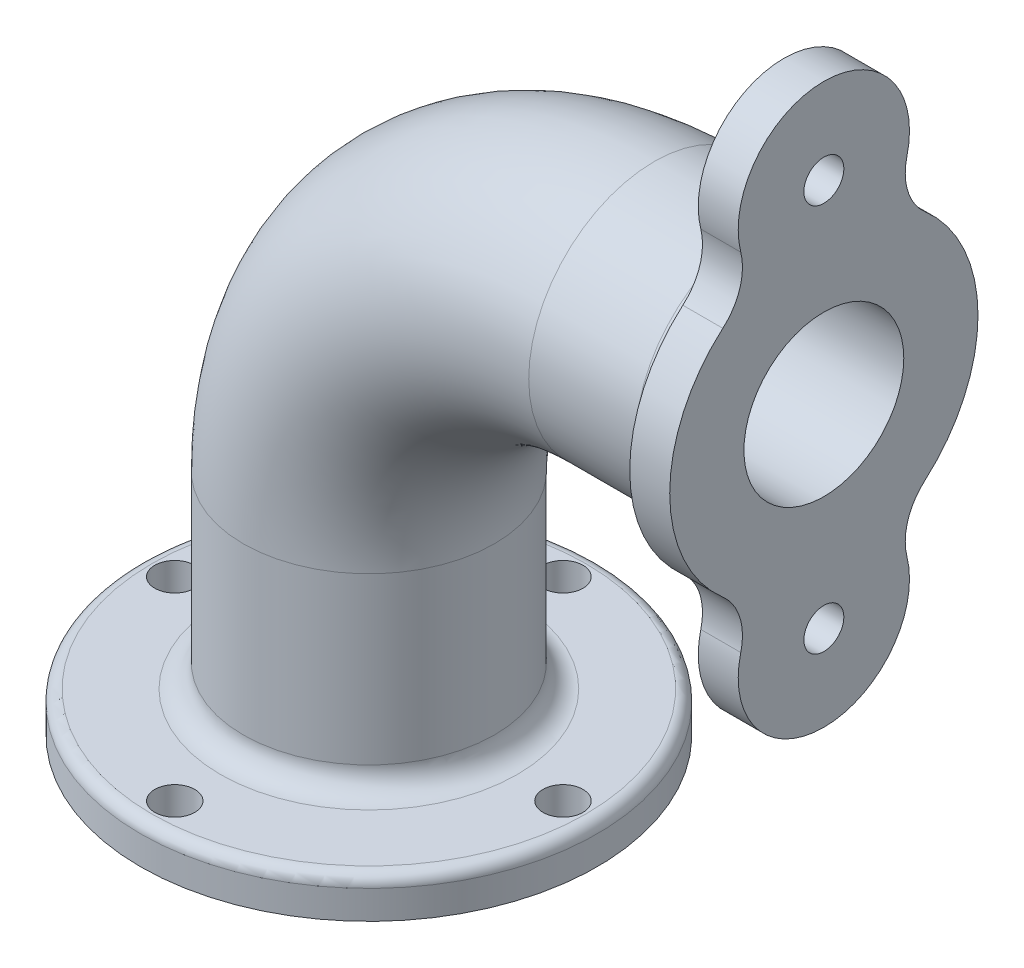
ISO-10303-21;
HEADER;
FILE_DESCRIPTION(('STEP AP214'),'2;1');
FILE_NAME('part.step','',(''),(''),'','','');
FILE_SCHEMA(('AUTOMOTIVE_DESIGN { 1 0 10303 214 1 1 1 1 }'));
ENDSEC;
DATA;
#1=APPLICATION_CONTEXT('core data for automotive mechanical design processes');
#2=APPLICATION_PROTOCOL_DEFINITION('international standard','automotive_design',2000,#1);
#3=PRODUCT_CONTEXT('',#1,'mechanical');
#4=PRODUCT('Part','Part','',(#3));
#5=PRODUCT_RELATED_PRODUCT_CATEGORY('part','',(#4));
#6=PRODUCT_DEFINITION_FORMATION('','',#4);
#7=PRODUCT_DEFINITION_CONTEXT('part definition',#1,'design');
#8=PRODUCT_DEFINITION('design','',#6,#7);
#9=PRODUCT_DEFINITION_SHAPE('','',#8);
#10=(LENGTH_UNIT() NAMED_UNIT(*) SI_UNIT(.MILLI.,.METRE.));
#11=(NAMED_UNIT(*) PLANE_ANGLE_UNIT() SI_UNIT($,.RADIAN.));
#12=(NAMED_UNIT(*) SI_UNIT($,.STERADIAN.) SOLID_ANGLE_UNIT());
#13=UNCERTAINTY_MEASURE_WITH_UNIT(LENGTH_MEASURE(1.E-05),#10,'distance_accuracy_value','');
#14=(GEOMETRIC_REPRESENTATION_CONTEXT(3) GLOBAL_UNCERTAINTY_ASSIGNED_CONTEXT((#13)) GLOBAL_UNIT_ASSIGNED_CONTEXT((#10,
#11,#12)) REPRESENTATION_CONTEXT('',''));
#15=CARTESIAN_POINT('',(0.,0.,0.));
#16=DIRECTION('',(0.,0.,1.));
#17=DIRECTION('',(1.,0.,0.));
#18=AXIS2_PLACEMENT_3D('',#15,#16,#17);
#19=CARTESIAN_POINT('',(-3.5,13.9705882352941,-12.1273519104486));
#20=DIRECTION('',(1.,0.,0.));
#21=DIRECTION('',(0.,0.,-1.));
#22=AXIS2_PLACEMENT_3D('',#19,#20,#21);
#23=PLANE('',#22);
#24=CARTESIAN_POINT('',(-3.5,0.,0.));
#25=DIRECTION('',(1.,0.,0.));
#26=DIRECTION('',(0.,0.,-1.));
#27=AXIS2_PLACEMENT_3D('',#24,#25,#26);
#28=CIRCLE('',#27,26.);
#29=CARTESIAN_POINT('',(-3.5,0.,-26.));
#30=VERTEX_POINT('',#29);
#31=EDGE_CURVE('E174',#30,#30,#28,.T.);
#32=ORIENTED_EDGE('',*,*,#31,.T.);
#33=EDGE_LOOP('',(#32));
#34=FACE_BOUND('',#33,.T.);
#35=CARTESIAN_POINT('',(-3.5,-34.,0.));
#36=DIRECTION('',(1.,0.,0.));
#37=DIRECTION('',(0.,0.,-1.));
#38=AXIS2_PLACEMENT_3D('',#35,#36,#37);
#39=CIRCLE('',#38,3.5);
#40=CARTESIAN_POINT('',(-3.5,-34.,-3.5));
#41=VERTEX_POINT('',#40);
#42=EDGE_CURVE('E218',#41,#41,#39,.T.);
#43=ORIENTED_EDGE('',*,*,#42,.T.);
#44=EDGE_LOOP('',(#43));
#45=FACE_BOUND('',#44,.T.);
#46=CARTESIAN_POINT('',(-3.5,34.,0.));
#47=DIRECTION('',(1.,0.,0.));
#48=DIRECTION('',(0.,0.,-1.));
#49=AXIS2_PLACEMENT_3D('',#46,#47,#48);
#50=CIRCLE('',#49,3.5);
#51=CARTESIAN_POINT('',(-3.5,34.,-3.5));
#52=VERTEX_POINT('',#51);
#53=EDGE_CURVE('E227',#52,#52,#50,.T.);
#54=ORIENTED_EDGE('',*,*,#53,.T.);
#55=EDGE_LOOP('',(#54));
#56=FACE_BOUND('',#55,.T.);
#57=CARTESIAN_POINT('',(-3.5,27.9411764705882,-24.2547038208972));
#58=DIRECTION('',(-1.,0.,0.));
#59=DIRECTION('',(0.,0.,-1.));
#60=AXIS2_PLACEMENT_3D('',#57,#58,#59);
#61=CIRCLE('',#60,10.);
#62=CARTESIAN_POINT('',(-3.5,20.389507154213,-17.699378463898));
#63=VERTEX_POINT('',#62);
#64=CARTESIAN_POINT('',(-3.5,30.3647058823529,-14.5528222925383));
#65=VERTEX_POINT('',#64);
#66=EDGE_CURVE('E145',#63,#65,#61,.T.);
#67=ORIENTED_EDGE('',*,*,#66,.F.);
#68=CARTESIAN_POINT('',(-3.5,0.,0.));
#69=DIRECTION('',(1.,0.,0.));
#70=DIRECTION('',(0.,0.,-1.));
#71=AXIS2_PLACEMENT_3D('',#68,#69,#70);
#72=CIRCLE('',#71,27.);
#73=CARTESIAN_POINT('',(-3.5,-20.389507154213,-17.699378463898));
#74=VERTEX_POINT('',#73);
#75=EDGE_CURVE('E95',#74,#63,#72,.T.);
#76=ORIENTED_EDGE('',*,*,#75,.F.);
#77=CARTESIAN_POINT('',(-3.5,-27.9411764705882,-24.2547038208972));
#78=DIRECTION('',(-1.,0.,0.));
#79=DIRECTION('',(0.,0.,-1.));
#80=AXIS2_PLACEMENT_3D('',#77,#78,#79);
#81=CIRCLE('',#80,10.);
#82=CARTESIAN_POINT('',(-3.5,-30.3647058823529,-14.5528222925383));
#83=VERTEX_POINT('',#82);
#84=EDGE_CURVE('E88',#83,#74,#81,.T.);
#85=ORIENTED_EDGE('',*,*,#84,.F.);
#86=CARTESIAN_POINT('',(-3.5,-34.,0.));
#87=DIRECTION('',(1.,0.,0.));
#88=DIRECTION('',(0.,0.,-1.));
#89=AXIS2_PLACEMENT_3D('',#86,#87,#88);
#90=CIRCLE('',#89,15.);
#91=CARTESIAN_POINT('',(-3.5,-30.3647058823529,14.5528222925383));
#92=VERTEX_POINT('',#91);
#93=EDGE_CURVE('E132',#92,#83,#90,.T.);
#94=ORIENTED_EDGE('',*,*,#93,.F.);
#95=CARTESIAN_POINT('',(-3.5,-27.9411764705882,24.2547038208972));
#96=DIRECTION('',(-1.,0.,0.));
#97=DIRECTION('',(0.,0.,-1.));
#98=AXIS2_PLACEMENT_3D('',#95,#96,#97);
#99=CIRCLE('',#98,10.);
#100=CARTESIAN_POINT('',(-3.5,-20.389507154213,17.699378463898));
#101=VERTEX_POINT('',#100);
#102=EDGE_CURVE('E152',#101,#92,#99,.T.);
#103=ORIENTED_EDGE('',*,*,#102,.F.);
#104=CARTESIAN_POINT('',(-3.5,0.,0.));
#105=DIRECTION('',(1.,0.,0.));
#106=DIRECTION('',(0.,0.,-1.));
#107=AXIS2_PLACEMENT_3D('',#104,#105,#106);
#108=CIRCLE('',#107,27.);
#109=CARTESIAN_POINT('',(-3.5,20.389507154213,17.699378463898));
#110=VERTEX_POINT('',#109);
#111=EDGE_CURVE('E148',#110,#101,#108,.T.);
#112=ORIENTED_EDGE('',*,*,#111,.F.);
#113=CARTESIAN_POINT('',(-3.5,27.9411764705882,24.2547038208972));
#114=DIRECTION('',(-1.,0.,0.));
#115=DIRECTION('',(0.,0.,1.));
#116=AXIS2_PLACEMENT_3D('',#113,#114,#115);
#117=CIRCLE('',#116,10.);
#118=CARTESIAN_POINT('',(-3.5,30.3647058823529,14.5528222925383));
#119=VERTEX_POINT('',#118);
#120=EDGE_CURVE('E149',#119,#110,#117,.T.);
#121=ORIENTED_EDGE('',*,*,#120,.F.);
#122=CARTESIAN_POINT('',(-3.5,34.,0.));
#123=DIRECTION('',(1.,0.,0.));
#124=DIRECTION('',(0.,0.,-1.));
#125=AXIS2_PLACEMENT_3D('',#122,#123,#124);
#126=CIRCLE('',#125,15.);
#127=EDGE_CURVE('E143',#65,#119,#126,.T.);
#128=ORIENTED_EDGE('',*,*,#127,.F.);
#129=EDGE_LOOP('',(#67,#76,#85,#94,#103,#112,#121,#128));
#130=FACE_BOUND('',#129,.T.);
#131=ADVANCED_FACE('F41',(#34,#45,#56,#130),#23,.F.);
#132=CARTESIAN_POINT('',(3.5,13.9705882352941,-12.1273519104486));
#133=DIRECTION('',(1.,0.,0.));
#134=DIRECTION('',(0.,0.,-1.));
#135=AXIS2_PLACEMENT_3D('',#132,#133,#134);
#136=PLANE('',#135);
#137=CARTESIAN_POINT('',(3.5,34.,0.));
#138=DIRECTION('',(1.,0.,0.));
#139=DIRECTION('',(0.,0.,-1.));
#140=AXIS2_PLACEMENT_3D('',#137,#138,#139);
#141=CIRCLE('',#140,3.5);
#142=CARTESIAN_POINT('',(3.5,34.,-3.5));
#143=VERTEX_POINT('',#142);
#144=EDGE_CURVE('E229',#143,#143,#141,.T.);
#145=ORIENTED_EDGE('',*,*,#144,.F.);
#146=EDGE_LOOP('',(#145));
#147=FACE_BOUND('',#146,.T.);
#148=CARTESIAN_POINT('',(3.5,27.9411764705882,-24.2547038208972));
#149=DIRECTION('',(-1.,0.,0.));
#150=DIRECTION('',(0.,0.,-1.));
#151=AXIS2_PLACEMENT_3D('',#148,#149,#150);
#152=CIRCLE('',#151,10.);
#153=CARTESIAN_POINT('',(3.5,20.389507154213,-17.699378463898));
#154=VERTEX_POINT('',#153);
#155=CARTESIAN_POINT('',(3.5,30.3647058823529,-14.5528222925383));
#156=VERTEX_POINT('',#155);
#157=EDGE_CURVE('E157',#154,#156,#152,.T.);
#158=ORIENTED_EDGE('',*,*,#157,.T.);
#159=CARTESIAN_POINT('',(3.5,34.,0.));
#160=DIRECTION('',(1.,0.,0.));
#161=DIRECTION('',(0.,0.,-1.));
#162=AXIS2_PLACEMENT_3D('',#159,#160,#161);
#163=CIRCLE('',#162,15.);
#164=CARTESIAN_POINT('',(3.5,30.3647058823529,14.5528222925383));
#165=VERTEX_POINT('',#164);
#166=EDGE_CURVE('E104',#156,#165,#163,.T.);
#167=ORIENTED_EDGE('',*,*,#166,.T.);
#168=CARTESIAN_POINT('',(3.5,27.9411764705882,24.2547038208972));
#169=DIRECTION('',(-1.,0.,0.));
#170=DIRECTION('',(0.,0.,1.));
#171=AXIS2_PLACEMENT_3D('',#168,#169,#170);
#172=CIRCLE('',#171,10.);
#173=CARTESIAN_POINT('',(3.5,20.389507154213,17.699378463898));
#174=VERTEX_POINT('',#173);
#175=EDGE_CURVE('E237',#165,#174,#172,.T.);
#176=ORIENTED_EDGE('',*,*,#175,.T.);
#177=CARTESIAN_POINT('',(3.5,0.,0.));
#178=DIRECTION('',(1.,0.,0.));
#179=DIRECTION('',(0.,0.,-1.));
#180=AXIS2_PLACEMENT_3D('',#177,#178,#179);
#181=CIRCLE('',#180,27.);
#182=CARTESIAN_POINT('',(3.5,-20.389507154213,17.699378463898));
#183=VERTEX_POINT('',#182);
#184=EDGE_CURVE('E241',#174,#183,#181,.T.);
#185=ORIENTED_EDGE('',*,*,#184,.T.);
#186=CARTESIAN_POINT('',(3.5,-27.9411764705882,24.2547038208972));
#187=DIRECTION('',(-1.,0.,0.));
#188=DIRECTION('',(0.,0.,-1.));
#189=AXIS2_PLACEMENT_3D('',#186,#187,#188);
#190=CIRCLE('',#189,10.);
#191=CARTESIAN_POINT('',(3.5,-30.3647058823529,14.5528222925383));
#192=VERTEX_POINT('',#191);
#193=EDGE_CURVE('E121',#183,#192,#190,.T.);
#194=ORIENTED_EDGE('',*,*,#193,.T.);
#195=CARTESIAN_POINT('',(3.5,-34.,0.));
#196=DIRECTION('',(1.,0.,0.));
#197=DIRECTION('',(0.,0.,-1.));
#198=AXIS2_PLACEMENT_3D('',#195,#196,#197);
#199=CIRCLE('',#198,15.);
#200=CARTESIAN_POINT('',(3.5,-30.3647058823529,-14.5528222925383));
#201=VERTEX_POINT('',#200);
#202=EDGE_CURVE('E120',#192,#201,#199,.T.);
#203=ORIENTED_EDGE('',*,*,#202,.T.);
#204=CARTESIAN_POINT('',(3.5,-27.9411764705882,-24.2547038208972));
#205=DIRECTION('',(-1.,0.,0.));
#206=DIRECTION('',(0.,0.,-1.));
#207=AXIS2_PLACEMENT_3D('',#204,#205,#206);
#208=CIRCLE('',#207,10.);
#209=CARTESIAN_POINT('',(3.5,-20.389507154213,-17.699378463898));
#210=VERTEX_POINT('',#209);
#211=EDGE_CURVE('E125',#201,#210,#208,.T.);
#212=ORIENTED_EDGE('',*,*,#211,.T.);
#213=CARTESIAN_POINT('',(3.5,0.,0.));
#214=DIRECTION('',(1.,0.,0.));
#215=DIRECTION('',(0.,0.,-1.));
#216=AXIS2_PLACEMENT_3D('',#213,#214,#215);
#217=CIRCLE('',#216,27.);
#218=EDGE_CURVE('E58',#210,#154,#217,.T.);
#219=ORIENTED_EDGE('',*,*,#218,.T.);
#220=EDGE_LOOP('',(#158,#167,#176,#185,#194,#203,#212,#219));
#221=FACE_BOUND('',#220,.T.);
#222=CARTESIAN_POINT('',(3.5,0.,0.));
#223=DIRECTION('',(1.,0.,0.));
#224=DIRECTION('',(0.,0.,-1.));
#225=AXIS2_PLACEMENT_3D('',#222,#223,#224);
#226=CIRCLE('',#225,14.);
#227=CARTESIAN_POINT('',(3.5,0.,-14.));
#228=VERTEX_POINT('',#227);
#229=EDGE_CURVE('E147',#228,#228,#226,.T.);
#230=ORIENTED_EDGE('',*,*,#229,.F.);
#231=EDGE_LOOP('',(#230));
#232=FACE_BOUND('',#231,.T.);
#233=CARTESIAN_POINT('',(3.5,-34.,0.));
#234=DIRECTION('',(1.,0.,0.));
#235=DIRECTION('',(0.,0.,-1.));
#236=AXIS2_PLACEMENT_3D('',#233,#234,#235);
#237=CIRCLE('',#236,3.5);
#238=CARTESIAN_POINT('',(3.5,-34.,-3.5));
#239=VERTEX_POINT('',#238);
#240=EDGE_CURVE('E223',#239,#239,#237,.T.);
#241=ORIENTED_EDGE('',*,*,#240,.F.);
#242=EDGE_LOOP('',(#241));
#243=FACE_BOUND('',#242,.T.);
#244=ADVANCED_FACE('F118',(#147,#221,#232,#243),#136,.T.);
#245=CARTESIAN_POINT('',(3.5,27.9411764705882,-24.2547038208972));
#246=DIRECTION('',(-1.,0.,0.));
#247=DIRECTION('',(0.,0.,1.));
#248=AXIS2_PLACEMENT_3D('',#245,#246,#247);
#249=CYLINDRICAL_SURFACE('',#248,10.);
#250=ORIENTED_EDGE('',*,*,#66,.T.);
#251=DIRECTION('',(-1.,0.,0.));
#252=VECTOR('',#251,1.);
#253=CARTESIAN_POINT('',(3.5,30.3647058823529,-14.5528222925383));
#254=LINE('',#253,#252);
#255=EDGE_CURVE('E167',#156,#65,#254,.T.);
#256=ORIENTED_EDGE('',*,*,#255,.F.);
#257=ORIENTED_EDGE('',*,*,#157,.F.);
#258=DIRECTION('',(-1.,0.,0.));
#259=VECTOR('',#258,1.);
#260=CARTESIAN_POINT('',(3.5,20.389507154213,-17.699378463898));
#261=LINE('',#260,#259);
#262=EDGE_CURVE('E139',#154,#63,#261,.T.);
#263=ORIENTED_EDGE('',*,*,#262,.T.);
#264=EDGE_LOOP('',(#250,#256,#257,#263));
#265=FACE_BOUND('',#264,.T.);
#266=ADVANCED_FACE('F260',(#265),#249,.F.);
#267=CARTESIAN_POINT('',(3.5,34.,0.));
#268=DIRECTION('',(-1.,0.,0.));
#269=DIRECTION('',(0.,0.,1.));
#270=AXIS2_PLACEMENT_3D('',#267,#268,#269);
#271=CYLINDRICAL_SURFACE('',#270,15.);
#272=ORIENTED_EDGE('',*,*,#127,.T.);
#273=DIRECTION('',(-1.,0.,0.));
#274=VECTOR('',#273,1.);
#275=CARTESIAN_POINT('',(3.5,30.3647058823529,14.5528222925383));
#276=LINE('',#275,#274);
#277=EDGE_CURVE('E170',#165,#119,#276,.T.);
#278=ORIENTED_EDGE('',*,*,#277,.F.);
#279=ORIENTED_EDGE('',*,*,#166,.F.);
#280=ORIENTED_EDGE('',*,*,#255,.T.);
#281=EDGE_LOOP('',(#272,#278,#279,#280));
#282=FACE_BOUND('',#281,.T.);
#283=ADVANCED_FACE('F382',(#282),#271,.T.);
#284=CARTESIAN_POINT('',(3.5,27.9411764705882,24.2547038208972));
#285=DIRECTION('',(-1.,0.,0.));
#286=DIRECTION('',(0.,0.,1.));
#287=AXIS2_PLACEMENT_3D('',#284,#285,#286);
#288=CYLINDRICAL_SURFACE('',#287,10.);
#289=ORIENTED_EDGE('',*,*,#120,.T.);
#290=DIRECTION('',(-1.,0.,0.));
#291=VECTOR('',#290,1.);
#292=CARTESIAN_POINT('',(3.5,20.389507154213,17.699378463898));
#293=LINE('',#292,#291);
#294=EDGE_CURVE('E165',#174,#110,#293,.T.);
#295=ORIENTED_EDGE('',*,*,#294,.F.);
#296=ORIENTED_EDGE('',*,*,#175,.F.);
#297=ORIENTED_EDGE('',*,*,#277,.T.);
#298=EDGE_LOOP('',(#289,#295,#296,#297));
#299=FACE_BOUND('',#298,.T.);
#300=ADVANCED_FACE('F381',(#299),#288,.F.);
#301=CARTESIAN_POINT('',(3.5,0.,0.));
#302=DIRECTION('',(-1.,0.,0.));
#303=DIRECTION('',(0.,0.,1.));
#304=AXIS2_PLACEMENT_3D('',#301,#302,#303);
#305=CYLINDRICAL_SURFACE('',#304,27.);
#306=ORIENTED_EDGE('',*,*,#111,.T.);
#307=DIRECTION('',(-1.,0.,0.));
#308=VECTOR('',#307,1.);
#309=CARTESIAN_POINT('',(3.5,-20.389507154213,17.699378463898));
#310=LINE('',#309,#308);
#311=EDGE_CURVE('E163',#183,#101,#310,.T.);
#312=ORIENTED_EDGE('',*,*,#311,.F.);
#313=ORIENTED_EDGE('',*,*,#184,.F.);
#314=ORIENTED_EDGE('',*,*,#294,.T.);
#315=EDGE_LOOP('',(#306,#312,#313,#314));
#316=FACE_BOUND('',#315,.T.);
#317=ADVANCED_FACE('F250',(#316),#305,.T.);
#318=CARTESIAN_POINT('',(3.5,-27.9411764705882,24.2547038208972));
#319=DIRECTION('',(-1.,0.,0.));
#320=DIRECTION('',(0.,0.,1.));
#321=AXIS2_PLACEMENT_3D('',#318,#319,#320);
#322=CYLINDRICAL_SURFACE('',#321,10.);
#323=ORIENTED_EDGE('',*,*,#102,.T.);
#324=DIRECTION('',(-1.,0.,0.));
#325=VECTOR('',#324,1.);
#326=CARTESIAN_POINT('',(3.5,-30.3647058823529,14.5528222925383));
#327=LINE('',#326,#325);
#328=EDGE_CURVE('E134',#192,#92,#327,.T.);
#329=ORIENTED_EDGE('',*,*,#328,.F.);
#330=ORIENTED_EDGE('',*,*,#193,.F.);
#331=ORIENTED_EDGE('',*,*,#311,.T.);
#332=EDGE_LOOP('',(#323,#329,#330,#331));
#333=FACE_BOUND('',#332,.T.);
#334=ADVANCED_FACE('F252',(#333),#322,.F.);
#335=CARTESIAN_POINT('',(3.5,-34.,0.));
#336=DIRECTION('',(-1.,0.,0.));
#337=DIRECTION('',(0.,0.,1.));
#338=AXIS2_PLACEMENT_3D('',#335,#336,#337);
#339=CYLINDRICAL_SURFACE('',#338,15.);
#340=ORIENTED_EDGE('',*,*,#93,.T.);
#341=DIRECTION('',(-1.,0.,0.));
#342=VECTOR('',#341,1.);
#343=CARTESIAN_POINT('',(3.5,-30.3647058823529,-14.5528222925383));
#344=LINE('',#343,#342);
#345=EDGE_CURVE('E126',#201,#83,#344,.T.);
#346=ORIENTED_EDGE('',*,*,#345,.F.);
#347=ORIENTED_EDGE('',*,*,#202,.F.);
#348=ORIENTED_EDGE('',*,*,#328,.T.);
#349=EDGE_LOOP('',(#340,#346,#347,#348));
#350=FACE_BOUND('',#349,.T.);
#351=ADVANCED_FACE('F128',(#350),#339,.T.);
#352=CARTESIAN_POINT('',(3.5,-27.9411764705882,-24.2547038208972));
#353=DIRECTION('',(-1.,0.,0.));
#354=DIRECTION('',(0.,0.,1.));
#355=AXIS2_PLACEMENT_3D('',#352,#353,#354);
#356=CYLINDRICAL_SURFACE('',#355,10.);
#357=ORIENTED_EDGE('',*,*,#84,.T.);
#358=DIRECTION('',(-1.,0.,0.));
#359=VECTOR('',#358,1.);
#360=CARTESIAN_POINT('',(3.5,-20.389507154213,-17.699378463898));
#361=LINE('',#360,#359);
#362=EDGE_CURVE('E133',#210,#74,#361,.T.);
#363=ORIENTED_EDGE('',*,*,#362,.F.);
#364=ORIENTED_EDGE('',*,*,#211,.F.);
#365=ORIENTED_EDGE('',*,*,#345,.T.);
#366=EDGE_LOOP('',(#357,#363,#364,#365));
#367=FACE_BOUND('',#366,.T.);
#368=ADVANCED_FACE('F136',(#367),#356,.F.);
#369=CARTESIAN_POINT('',(3.5,0.,0.));
#370=DIRECTION('',(-1.,0.,0.));
#371=DIRECTION('',(0.,0.,1.));
#372=AXIS2_PLACEMENT_3D('',#369,#370,#371);
#373=CYLINDRICAL_SURFACE('',#372,27.);
#374=ORIENTED_EDGE('',*,*,#75,.T.);
#375=ORIENTED_EDGE('',*,*,#262,.F.);
#376=ORIENTED_EDGE('',*,*,#218,.F.);
#377=ORIENTED_EDGE('',*,*,#362,.T.);
#378=EDGE_LOOP('',(#374,#375,#376,#377));
#379=FACE_BOUND('',#378,.T.);
#380=ADVANCED_FACE('F256',(#379),#373,.T.);
#381=CARTESIAN_POINT('',(3.5,0.,0.));
#382=DIRECTION('',(-1.,0.,0.));
#383=DIRECTION('',(0.,0.,1.));
#384=AXIS2_PLACEMENT_3D('',#381,#382,#383);
#385=CYLINDRICAL_SURFACE('',#384,14.);
#386=ORIENTED_EDGE('',*,*,#229,.T.);
#387=EDGE_LOOP('',(#386));
#388=FACE_BOUND('',#387,.T.);
#389=CARTESIAN_POINT('',(-26.1956432875197,0.,0.));
#390=DIRECTION('',(1.,0.,0.));
#391=DIRECTION('',(0.,0.,1.));
#392=AXIS2_PLACEMENT_3D('',#389,#390,#391);
#393=CIRCLE('',#392,14.);
#394=CARTESIAN_POINT('',(-26.1956432875197,14.,0.));
#395=VERTEX_POINT('',#394);
#396=EDGE_CURVE('E215',#395,#395,#393,.F.);
#397=ORIENTED_EDGE('',*,*,#396,.T.);
#398=EDGE_LOOP('',(#397));
#399=FACE_BOUND('',#398,.T.);
#400=ADVANCED_FACE('F261',(#388,#399),#385,.F.);
#401=CARTESIAN_POINT('',(3.5,34.,0.));
#402=DIRECTION('',(-1.,0.,0.));
#403=DIRECTION('',(0.,0.,1.));
#404=AXIS2_PLACEMENT_3D('',#401,#402,#403);
#405=CYLINDRICAL_SURFACE('',#404,3.5);
#406=ORIENTED_EDGE('',*,*,#144,.T.);
#407=EDGE_LOOP('',(#406));
#408=FACE_BOUND('',#407,.T.);
#409=ORIENTED_EDGE('',*,*,#53,.F.);
#410=EDGE_LOOP('',(#409));
#411=FACE_BOUND('',#410,.T.);
#412=ADVANCED_FACE('F269',(#408,#411),#405,.F.);
#413=CARTESIAN_POINT('',(3.5,-34.,0.));
#414=DIRECTION('',(-1.,0.,0.));
#415=DIRECTION('',(0.,0.,1.));
#416=AXIS2_PLACEMENT_3D('',#413,#414,#415);
#417=CYLINDRICAL_SURFACE('',#416,3.5);
#418=ORIENTED_EDGE('',*,*,#240,.T.);
#419=EDGE_LOOP('',(#418));
#420=FACE_BOUND('',#419,.T.);
#421=ORIENTED_EDGE('',*,*,#42,.F.);
#422=EDGE_LOOP('',(#421));
#423=FACE_BOUND('',#422,.T.);
#424=ADVANCED_FACE('F285',(#420,#423),#417,.F.);
#425=CARTESIAN_POINT('',(0.,0.,0.));
#426=DIRECTION('',(-1.,0.,0.));
#427=DIRECTION('',(0.,0.,1.));
#428=AXIS2_PLACEMENT_3D('',#425,#426,#427);
#429=CYLINDRICAL_SURFACE('',#428,22.);
#430=CARTESIAN_POINT('',(-7.5,0.,0.));
#431=DIRECTION('',(1.,0.,0.));
#432=DIRECTION('',(0.,0.,-1.));
#433=AXIS2_PLACEMENT_3D('',#430,#431,#432);
#434=CIRCLE('',#433,22.);
#435=CARTESIAN_POINT('',(-7.5,0.,-22.));
#436=VERTEX_POINT('',#435);
#437=EDGE_CURVE('E175',#436,#436,#434,.F.);
#438=ORIENTED_EDGE('',*,*,#437,.T.);
#439=EDGE_LOOP('',(#438));
#440=FACE_BOUND('',#439,.T.);
#441=CARTESIAN_POINT('',(-26.1956432875197,0.,0.));
#442=DIRECTION('',(1.,0.,0.));
#443=DIRECTION('',(0.,0.,1.));
#444=AXIS2_PLACEMENT_3D('',#441,#442,#443);
#445=CIRCLE('',#444,22.);
#446=CARTESIAN_POINT('',(-26.1956432875197,22.,0.));
#447=VERTEX_POINT('',#446);
#448=EDGE_CURVE('E207',#447,#447,#445,.T.);
#449=ORIENTED_EDGE('',*,*,#448,.T.);
#450=EDGE_LOOP('',(#449));
#451=FACE_BOUND('',#450,.T.);
#452=ADVANCED_FACE('F288',(#440,#451),#429,.T.);
#453=CARTESIAN_POINT('',(-26.1956432875197,-50.,0.));
#454=DIRECTION('',(0.,0.,1.));
#455=DIRECTION('',(1.,0.,0.));
#456=AXIS2_PLACEMENT_3D('',#453,#454,#455);
#457=TOROIDAL_SURFACE('',#456,50.,22.);
#458=CARTESIAN_POINT('',(-76.1956432875197,-50.,0.));
#459=DIRECTION('',(0.,1.,0.));
#460=DIRECTION('',(0.,0.,1.));
#461=AXIS2_PLACEMENT_3D('',#458,#459,#460);
#462=CIRCLE('',#461,22.);
#463=CARTESIAN_POINT('',(-98.1956432875197,-50.,0.));
#464=VERTEX_POINT('',#463);
#465=EDGE_CURVE('E216',#464,#464,#462,.T.);
#466=CARTESIAN_POINT('',(-26.1956432875197,-50.,0.));
#467=DIRECTION('',(0.,0.,1.));
#468=DIRECTION('',(1.,0.,0.));
#469=AXIS2_PLACEMENT_3D('',#466,#467,#468);
#470=CIRCLE('',#469,72.);
#471=EDGE_CURVE('',#447,#464,#470,.T.);
#472=ORIENTED_EDGE('',*,*,#448,.F.);
#473=ORIENTED_EDGE('',*,*,#465,.T.);
#474=ORIENTED_EDGE('',*,*,#471,.T.);
#475=ORIENTED_EDGE('',*,*,#471,.F.);
#476=EDGE_LOOP('',(#472,#474,#473,#475));
#477=FACE_BOUND('',#476,.T.);
#478=ADVANCED_FACE('F294',(#477),#457,.T.);
#479=CARTESIAN_POINT('',(-76.1956432875197,-50.,0.));
#480=DIRECTION('',(0.,-1.,0.));
#481=DIRECTION('',(0.,0.,-1.));
#482=AXIS2_PLACEMENT_3D('',#479,#480,#481);
#483=CYLINDRICAL_SURFACE('',#482,22.);
#484=CARTESIAN_POINT('',(-76.1956432875197,-79.,0.));
#485=DIRECTION('',(0.,-1.,0.));
#486=DIRECTION('',(0.,0.,-1.));
#487=AXIS2_PLACEMENT_3D('',#484,#485,#486);
#488=CIRCLE('',#487,22.);
#489=CARTESIAN_POINT('',(-76.1956432875197,-79.,-22.));
#490=VERTEX_POINT('',#489);
#491=EDGE_CURVE('E178',#490,#490,#488,.F.);
#492=ORIENTED_EDGE('',*,*,#491,.T.);
#493=EDGE_LOOP('',(#492));
#494=FACE_BOUND('',#493,.T.);
#495=ORIENTED_EDGE('',*,*,#465,.F.);
#496=EDGE_LOOP('',(#495));
#497=FACE_BOUND('',#496,.T.);
#498=ADVANCED_FACE('F293',(#494,#497),#483,.T.);
#499=CARTESIAN_POINT('',(-26.1956432875197,-50.,0.));
#500=DIRECTION('',(0.,0.,1.));
#501=DIRECTION('',(1.,0.,0.));
#502=AXIS2_PLACEMENT_3D('',#499,#500,#501);
#503=TOROIDAL_SURFACE('',#502,50.,14.);
#504=CARTESIAN_POINT('',(-76.1956432875197,-50.,0.));
#505=DIRECTION('',(0.,1.,0.));
#506=DIRECTION('',(0.,0.,1.));
#507=AXIS2_PLACEMENT_3D('',#504,#505,#506);
#508=CIRCLE('',#507,14.);
#509=CARTESIAN_POINT('',(-90.1956432875197,-50.,0.));
#510=VERTEX_POINT('',#509);
#511=EDGE_CURVE('E213',#510,#510,#508,.F.);
#512=CARTESIAN_POINT('',(-26.1956432875197,-50.,0.));
#513=DIRECTION('',(0.,0.,1.));
#514=DIRECTION('',(1.,0.,0.));
#515=AXIS2_PLACEMENT_3D('',#512,#513,#514);
#516=CIRCLE('',#515,64.);
#517=EDGE_CURVE('',#395,#510,#516,.T.);
#518=ORIENTED_EDGE('',*,*,#396,.F.);
#519=ORIENTED_EDGE('',*,*,#511,.T.);
#520=ORIENTED_EDGE('',*,*,#517,.T.);
#521=ORIENTED_EDGE('',*,*,#517,.F.);
#522=EDGE_LOOP('',(#518,#520,#519,#521));
#523=FACE_BOUND('',#522,.T.);
#524=ADVANCED_FACE('F295',(#523),#503,.F.);
#525=CARTESIAN_POINT('',(-76.1956432875197,-50.,0.));
#526=DIRECTION('',(0.,-1.,0.));
#527=DIRECTION('',(0.,0.,-1.));
#528=AXIS2_PLACEMENT_3D('',#525,#526,#527);
#529=CYLINDRICAL_SURFACE('',#528,14.);
#530=ORIENTED_EDGE('',*,*,#511,.F.);
#531=EDGE_LOOP('',(#530));
#532=FACE_BOUND('',#531,.T.);
#533=CARTESIAN_POINT('',(-76.1956432875197,-90.,0.));
#534=DIRECTION('',(0.,-1.,0.));
#535=DIRECTION('',(0.,0.,-1.));
#536=AXIS2_PLACEMENT_3D('',#533,#534,#535);
#537=CIRCLE('',#536,14.);
#538=CARTESIAN_POINT('',(-76.1956432875197,-90.,-14.));
#539=VERTEX_POINT('',#538);
#540=EDGE_CURVE('E197',#539,#539,#537,.T.);
#541=ORIENTED_EDGE('',*,*,#540,.T.);
#542=EDGE_LOOP('',(#541));
#543=FACE_BOUND('',#542,.T.);
#544=ADVANCED_FACE('F303',(#532,#543),#529,.F.);
#545=CARTESIAN_POINT('',(-76.1956432875197,-90.,0.));
#546=DIRECTION('',(0.,-1.,0.));
#547=DIRECTION('',(0.,0.,-1.));
#548=AXIS2_PLACEMENT_3D('',#545,#546,#547);
#549=PLANE('',#548);
#550=CARTESIAN_POINT('',(-110.19564328752,-90.,0.));
#551=DIRECTION('',(0.,-1.,0.));
#552=DIRECTION('',(0.,0.,-1.));
#553=AXIS2_PLACEMENT_3D('',#550,#551,#552);
#554=CIRCLE('',#553,3.50000000000001);
#555=CARTESIAN_POINT('',(-110.19564328752,-90.,-3.50000000000002));
#556=VERTEX_POINT('',#555);
#557=EDGE_CURVE('E188',#556,#556,#554,.T.);
#558=ORIENTED_EDGE('',*,*,#557,.F.);
#559=EDGE_LOOP('',(#558));
#560=FACE_BOUND('',#559,.T.);
#561=CARTESIAN_POINT('',(-42.1956432875197,-90.,0.));
#562=DIRECTION('',(0.,-1.,0.));
#563=DIRECTION('',(0.,0.,-1.));
#564=AXIS2_PLACEMENT_3D('',#561,#562,#563);
#565=CIRCLE('',#564,3.5);
#566=CARTESIAN_POINT('',(-42.1956432875197,-90.,-3.50000000000001));
#567=VERTEX_POINT('',#566);
#568=EDGE_CURVE('E338',#567,#567,#565,.T.);
#569=ORIENTED_EDGE('',*,*,#568,.F.);
#570=EDGE_LOOP('',(#569));
#571=FACE_BOUND('',#570,.T.);
#572=CARTESIAN_POINT('',(-76.1956432875197,-90.,34.));
#573=DIRECTION('',(0.,-1.,0.));
#574=DIRECTION('',(0.,0.,-1.));
#575=AXIS2_PLACEMENT_3D('',#572,#573,#574);
#576=CIRCLE('',#575,3.50000000000001);
#577=CARTESIAN_POINT('',(-76.1956432875197,-90.,30.5));
#578=VERTEX_POINT('',#577);
#579=EDGE_CURVE('E344',#578,#578,#576,.T.);
#580=ORIENTED_EDGE('',*,*,#579,.F.);
#581=EDGE_LOOP('',(#580));
#582=FACE_BOUND('',#581,.T.);
#583=CARTESIAN_POINT('',(-76.1956432875197,-90.,-34.));
#584=DIRECTION('',(0.,-1.,0.));
#585=DIRECTION('',(0.,0.,-1.));
#586=AXIS2_PLACEMENT_3D('',#583,#584,#585);
#587=CIRCLE('',#586,3.50000000000001);
#588=CARTESIAN_POINT('',(-76.1956432875197,-90.,-37.5));
#589=VERTEX_POINT('',#588);
#590=EDGE_CURVE('E209',#589,#589,#587,.T.);
#591=ORIENTED_EDGE('',*,*,#590,.F.);
#592=EDGE_LOOP('',(#591));
#593=FACE_BOUND('',#592,.T.);
#594=CARTESIAN_POINT('',(-76.1956432875197,-90.,0.));
#595=DIRECTION('',(0.,-1.,0.));
#596=DIRECTION('',(0.,0.,-1.));
#597=AXIS2_PLACEMENT_3D('',#594,#595,#596);
#598=CIRCLE('',#597,40.);
#599=CARTESIAN_POINT('',(-76.1956432875197,-90.,-40.));
#600=VERTEX_POINT('',#599);
#601=EDGE_CURVE('E201',#600,#600,#598,.T.);
#602=ORIENTED_EDGE('',*,*,#601,.T.);
#603=EDGE_LOOP('',(#602));
#604=FACE_BOUND('',#603,.T.);
#605=ORIENTED_EDGE('',*,*,#540,.F.);
#606=EDGE_LOOP('',(#605));
#607=FACE_BOUND('',#606,.T.);
#608=ADVANCED_FACE('F297',(#560,#571,#582,#593,#604,#607),#549,.T.);
#609=CARTESIAN_POINT('',(-76.1956432875197,-83.,0.));
#610=DIRECTION('',(0.,-1.,0.));
#611=DIRECTION('',(0.,0.,-1.));
#612=AXIS2_PLACEMENT_3D('',#609,#610,#611);
#613=PLANE('',#612);
#614=CARTESIAN_POINT('',(-110.19564328752,-83.,0.));
#615=DIRECTION('',(0.,-1.,0.));
#616=DIRECTION('',(0.,0.,-1.));
#617=AXIS2_PLACEMENT_3D('',#614,#615,#616);
#618=CIRCLE('',#617,3.50000000000001);
#619=CARTESIAN_POINT('',(-110.19564328752,-83.,-3.50000000000002));
#620=VERTEX_POINT('',#619);
#621=EDGE_CURVE('E44',#620,#620,#618,.T.);
#622=ORIENTED_EDGE('',*,*,#621,.T.);
#623=EDGE_LOOP('',(#622));
#624=FACE_BOUND('',#623,.T.);
#625=CARTESIAN_POINT('',(-42.1956432875197,-83.,0.));
#626=DIRECTION('',(0.,-1.,0.));
#627=DIRECTION('',(0.,0.,-1.));
#628=AXIS2_PLACEMENT_3D('',#625,#626,#627);
#629=CIRCLE('',#628,3.5);
#630=CARTESIAN_POINT('',(-42.1956432875197,-83.,-3.50000000000001));
#631=VERTEX_POINT('',#630);
#632=EDGE_CURVE('E195',#631,#631,#629,.T.);
#633=ORIENTED_EDGE('',*,*,#632,.T.);
#634=EDGE_LOOP('',(#633));
#635=FACE_BOUND('',#634,.T.);
#636=CARTESIAN_POINT('',(-76.1956432875197,-83.,34.));
#637=DIRECTION('',(0.,-1.,0.));
#638=DIRECTION('',(0.,0.,-1.));
#639=AXIS2_PLACEMENT_3D('',#636,#637,#638);
#640=CIRCLE('',#639,3.50000000000001);
#641=CARTESIAN_POINT('',(-76.1956432875197,-83.,30.5));
#642=VERTEX_POINT('',#641);
#643=EDGE_CURVE('E186',#642,#642,#640,.T.);
#644=ORIENTED_EDGE('',*,*,#643,.T.);
#645=EDGE_LOOP('',(#644));
#646=FACE_BOUND('',#645,.T.);
#647=CARTESIAN_POINT('',(-76.1956432875197,-83.,-34.));
#648=DIRECTION('',(0.,-1.,0.));
#649=DIRECTION('',(0.,0.,-1.));
#650=AXIS2_PLACEMENT_3D('',#647,#648,#649);
#651=CIRCLE('',#650,3.50000000000001);
#652=CARTESIAN_POINT('',(-76.1956432875197,-83.,-37.5));
#653=VERTEX_POINT('',#652);
#654=EDGE_CURVE('E187',#653,#653,#651,.T.);
#655=ORIENTED_EDGE('',*,*,#654,.T.);
#656=EDGE_LOOP('',(#655));
#657=FACE_BOUND('',#656,.T.);
#658=CARTESIAN_POINT('',(-76.1956432875197,-83.,0.));
#659=DIRECTION('',(0.,-1.,0.));
#660=DIRECTION('',(0.,0.,-1.));
#661=AXIS2_PLACEMENT_3D('',#658,#659,#660);
#662=CIRCLE('',#661,38.);
#663=CARTESIAN_POINT('',(-76.1956432875197,-83.,-38.));
#664=VERTEX_POINT('',#663);
#665=EDGE_CURVE('E11',#664,#664,#662,.F.);
#666=ORIENTED_EDGE('',*,*,#665,.T.);
#667=EDGE_LOOP('',(#666));
#668=FACE_BOUND('',#667,.T.);
#669=CARTESIAN_POINT('',(-76.1956432875197,-83.,0.));
#670=DIRECTION('',(0.,-1.,0.));
#671=DIRECTION('',(0.,0.,-1.));
#672=AXIS2_PLACEMENT_3D('',#669,#670,#671);
#673=CIRCLE('',#672,26.);
#674=CARTESIAN_POINT('',(-76.1956432875197,-83.,-26.));
#675=VERTEX_POINT('',#674);
#676=EDGE_CURVE('E181',#675,#675,#673,.T.);
#677=ORIENTED_EDGE('',*,*,#676,.T.);
#678=EDGE_LOOP('',(#677));
#679=FACE_BOUND('',#678,.T.);
#680=ADVANCED_FACE('F312',(#624,#635,#646,#657,#668,#679),#613,.F.);
#681=CARTESIAN_POINT('',(-76.1956432875197,-90.,0.));
#682=DIRECTION('',(0.,1.,0.));
#683=DIRECTION('',(0.,0.,1.));
#684=AXIS2_PLACEMENT_3D('',#681,#682,#683);
#685=CYLINDRICAL_SURFACE('',#684,40.);
#686=CARTESIAN_POINT('',(-76.1956432875197,-85.,0.));
#687=DIRECTION('',(0.,-1.,0.));
#688=DIRECTION('',(0.,0.,-1.));
#689=AXIS2_PLACEMENT_3D('',#686,#687,#688);
#690=CIRCLE('',#689,40.);
#691=CARTESIAN_POINT('',(-76.1956432875197,-85.,-40.));
#692=VERTEX_POINT('',#691);
#693=EDGE_CURVE('E51',#692,#692,#690,.T.);
#694=ORIENTED_EDGE('',*,*,#693,.T.);
#695=EDGE_LOOP('',(#694));
#696=FACE_BOUND('',#695,.T.);
#697=ORIENTED_EDGE('',*,*,#601,.F.);
#698=EDGE_LOOP('',(#697));
#699=FACE_BOUND('',#698,.T.);
#700=ADVANCED_FACE('F307',(#696,#699),#685,.T.);
#701=CARTESIAN_POINT('',(-7.5,0.,0.));
#702=DIRECTION('',(1.,0.,0.));
#703=DIRECTION('',(0.,0.,-1.));
#704=AXIS2_PLACEMENT_3D('',#701,#702,#703);
#705=TOROIDAL_SURFACE('',#704,26.,4.);
#706=ORIENTED_EDGE('',*,*,#31,.F.);
#707=EDGE_LOOP('',(#706));
#708=FACE_BOUND('',#707,.T.);
#709=ORIENTED_EDGE('',*,*,#437,.F.);
#710=EDGE_LOOP('',(#709));
#711=FACE_BOUND('',#710,.T.);
#712=ADVANCED_FACE('F315',(#708,#711),#705,.F.);
#713=CARTESIAN_POINT('',(-76.1956432875197,-79.,0.));
#714=DIRECTION('',(0.,-1.,0.));
#715=DIRECTION('',(0.,0.,-1.));
#716=AXIS2_PLACEMENT_3D('',#713,#714,#715);
#717=TOROIDAL_SURFACE('',#716,26.,4.);
#718=ORIENTED_EDGE('',*,*,#676,.F.);
#719=EDGE_LOOP('',(#718));
#720=FACE_BOUND('',#719,.T.);
#721=ORIENTED_EDGE('',*,*,#491,.F.);
#722=EDGE_LOOP('',(#721));
#723=FACE_BOUND('',#722,.T.);
#724=ADVANCED_FACE('F365',(#720,#723),#717,.F.);
#725=CARTESIAN_POINT('',(-76.1956432875197,-85.,0.));
#726=DIRECTION('',(0.,-1.,0.));
#727=DIRECTION('',(0.,0.,-1.));
#728=AXIS2_PLACEMENT_3D('',#725,#726,#727);
#729=TOROIDAL_SURFACE('',#728,38.,2.);
#730=ORIENTED_EDGE('',*,*,#665,.F.);
#731=EDGE_LOOP('',(#730));
#732=FACE_BOUND('',#731,.T.);
#733=ORIENTED_EDGE('',*,*,#693,.F.);
#734=EDGE_LOOP('',(#733));
#735=FACE_BOUND('',#734,.T.);
#736=ADVANCED_FACE('F43',(#732,#735),#729,.T.);
#737=CARTESIAN_POINT('',(-76.1956432875197,-80.,-34.));
#738=DIRECTION('',(0.,-1.,0.));
#739=DIRECTION('',(0.,0.,-1.));
#740=AXIS2_PLACEMENT_3D('',#737,#738,#739);
#741=CYLINDRICAL_SURFACE('',#740,3.50000000000001);
#742=ORIENTED_EDGE('',*,*,#590,.T.);
#743=EDGE_LOOP('',(#742));
#744=FACE_BOUND('',#743,.T.);
#745=ORIENTED_EDGE('',*,*,#654,.F.);
#746=EDGE_LOOP('',(#745));
#747=FACE_BOUND('',#746,.T.);
#748=ADVANCED_FACE('F318',(#744,#747),#741,.F.);
#749=CARTESIAN_POINT('',(-76.1956432875197,-80.,34.));
#750=DIRECTION('',(0.,-1.,0.));
#751=DIRECTION('',(0.,0.,-1.));
#752=AXIS2_PLACEMENT_3D('',#749,#750,#751);
#753=CYLINDRICAL_SURFACE('',#752,3.50000000000001);
#754=ORIENTED_EDGE('',*,*,#579,.T.);
#755=EDGE_LOOP('',(#754));
#756=FACE_BOUND('',#755,.T.);
#757=ORIENTED_EDGE('',*,*,#643,.F.);
#758=EDGE_LOOP('',(#757));
#759=FACE_BOUND('',#758,.T.);
#760=ADVANCED_FACE('F324',(#756,#759),#753,.F.);
#761=CARTESIAN_POINT('',(-42.1956432875197,-80.,0.));
#762=DIRECTION('',(0.,-1.,0.));
#763=DIRECTION('',(0.,0.,-1.));
#764=AXIS2_PLACEMENT_3D('',#761,#762,#763);
#765=CYLINDRICAL_SURFACE('',#764,3.5);
#766=ORIENTED_EDGE('',*,*,#568,.T.);
#767=EDGE_LOOP('',(#766));
#768=FACE_BOUND('',#767,.T.);
#769=ORIENTED_EDGE('',*,*,#632,.F.);
#770=EDGE_LOOP('',(#769));
#771=FACE_BOUND('',#770,.T.);
#772=ADVANCED_FACE('F327',(#768,#771),#765,.F.);
#773=CARTESIAN_POINT('',(-110.19564328752,-80.,0.));
#774=DIRECTION('',(0.,-1.,0.));
#775=DIRECTION('',(0.,0.,-1.));
#776=AXIS2_PLACEMENT_3D('',#773,#774,#775);
#777=CYLINDRICAL_SURFACE('',#776,3.50000000000001);
#778=ORIENTED_EDGE('',*,*,#557,.T.);
#779=EDGE_LOOP('',(#778));
#780=FACE_BOUND('',#779,.T.);
#781=ORIENTED_EDGE('',*,*,#621,.F.);
#782=EDGE_LOOP('',(#781));
#783=FACE_BOUND('',#782,.T.);
#784=ADVANCED_FACE('F331',(#780,#783),#777,.F.);
#785=CLOSED_SHELL('',(#131,#244,#266,#283,#300,#317,#334,#351,#368,#380,#400,#412,#424,#452,
#478,#498,#524,#544,#608,#680,#700,#712,#724,#736,#748,#760,#772,#784));
#786=MANIFOLD_SOLID_BREP('B2',#785);
#787=ADVANCED_BREP_SHAPE_REPRESENTATION('',(#18,#786),#14);
#788=SHAPE_DEFINITION_REPRESENTATION(#9,#787);
ENDSEC;
END-ISO-10303-21;
